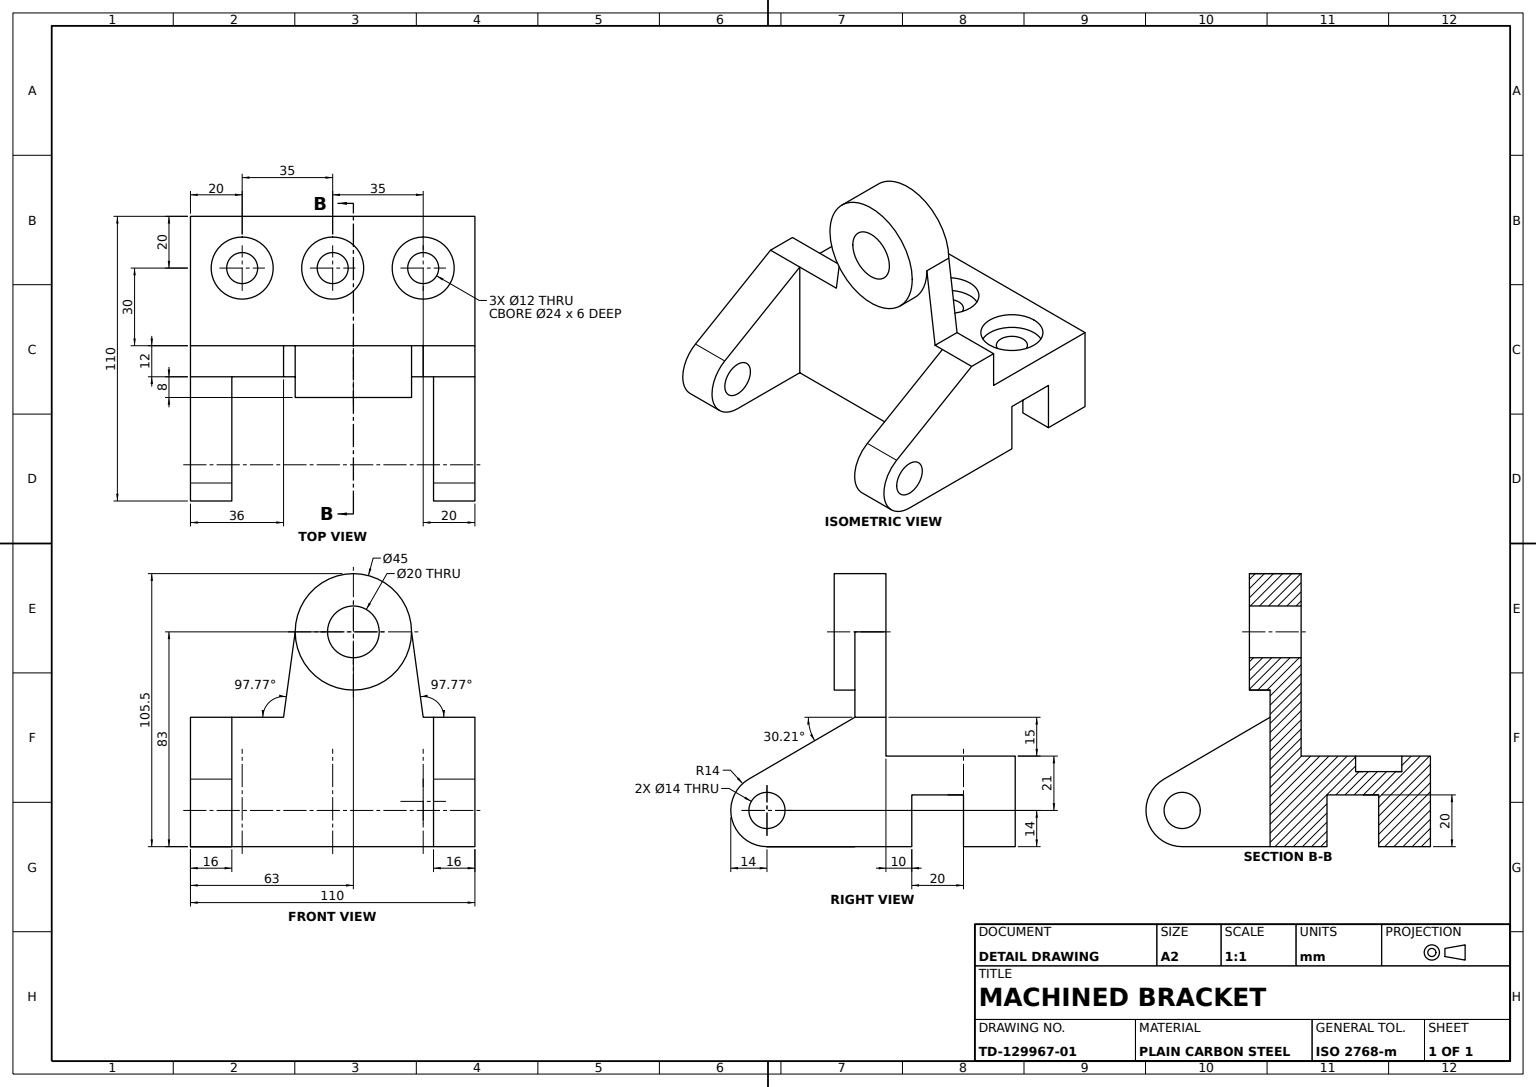
from build123d import *

# Parameters (mm, degrees)
SIDE_ARM_16MM_DEPTH          = 16
BRACKET_BODY_94MM_DEPTH      = 94
SECOND_START                 = -16
SECOND_ARM_16MM_DEPTH        = 16
PIVOT_HOLE_SKETCH_14_R       = 7
PIVOT_HOLES_14_THROUGH_DEPTH = 231
BEARING_BOSS_45_DEPTH        = 8
BEARING_BOSS_45_DEPTH_BACK   = 12
BEARING_BOSS_SKETCH_45_R     = 22.5
BOSS_SUPPORT_WEB_12MM_DEPTH  = 12
BEARING_BORE_SKETCH_20_R     = 10
BEARING_BORE_20_DEPTH        = 101
COUNTERBORE_SKETCH_24_R      = 12
COUNTERBORES_24X6_DEPTH      = 6
MOUNTING_HOLE_SKETCH_12_R    = 6
MOUNTING_HOLES_12_DEPTH      = 58


with BuildPart() as part:
    # Side Arm Profile → Side Arm 16mm (new body)
    with BuildSketch(Plane(origin=(0, 0, 0), x_dir=(0, 0, -1), z_dir=(1, 0, 0))):
        with BuildLine():
            Line((0, 0), (-20, 0))
            Line((-20, 0), (-20, 20))
            Line((-20, 20), (-40, 20))
            Line((-40, 20), (-40, 0))
            Line((-40, 0), (-96, 0))
            ThreePointArc((-96, 0), (-109.516186166, 10.351341133), (-103.045136072, 26.098184068))
            Line((-103.045136072, 26.098184068), (-62, 50))
            Line((-62, 50), (-50, 50))
            Line((-50, 50), (-50, 35))
            Line((-50, 35), (0, 35))
            Line((0, 35), (0, 0))
        make_face()
    extrude(amount=-SIDE_ARM_16MM_DEPTH)

    # Bracket Body Profile → Bracket Body 94mm (add)
    with BuildSketch(Plane.ZY.offset(16)):
        Polygon((0, 0), (0, 35), (50, 35), (50, 50), (62, 50), (62, 0), (40, 0), (40, 20), (20, 20), (20, 0), align=None)
    extrude(amount=BRACKET_BODY_94MM_DEPTH)

    # Second Arm Profile → Second Arm 16mm (add)
    with BuildSketch(Plane.ZY.offset(110).offset(SECOND_START)):
        with BuildLine():
            Line((62, 0), (62, 50))
            Line((62, 50), (103.045136072, 26.098184068))
            ThreePointArc((103.045136072, 26.098184068), (109.516186166, 10.351341133), (96, 0))
            Line((96, 0), (62, 0))
        make_face()
    extrude(amount=SECOND_ARM_16MM_DEPTH)

    # Pivot Hole Sketch Ø14 → Pivot Holes Ø14 Through (cut)
    with BuildSketch(Plane(origin=(0, 0, 0), x_dir=(0, 0, -1), z_dir=(1, 0, 0))):
        with Locations((-96, 14)):
            Circle(PIVOT_HOLE_SKETCH_14_R)
    extrude(amount=-PIVOT_HOLES_14_THROUGH_DEPTH, mode=Mode.SUBTRACT)



with BuildPart() as body_2:
    # Bearing Boss Sketch Ø45 → Bearing Boss Ø45 (new, two sides: drawn at the far end of the back side and taken through both)
    with BuildSketch(Plane.XY.offset(62).offset(-BEARING_BOSS_45_DEPTH_BACK)):
        with Locations((-47, 83)):
            Circle(BEARING_BOSS_SKETCH_45_R)
    extrude(amount=BEARING_BOSS_45_DEPTH + BEARING_BOSS_45_DEPTH_BACK)


with BuildPart() as part_1:
    add(part.part)

    add(body_2.part)  # Boss Support Web 12mm merges body 2
    # Boss Support Web Profile → Boss Support Web 12mm (add)
    with BuildSketch(Plane.XY.offset(62)):
        with BuildLine():
            Line((-20, 50), (-24.5, 83))
            ThreePointArc((-24.5, 83), (-47, 60.5), (-69.5, 83))
            Line((-69.5, 83), (-74, 50))
            Line((-74, 50), (-20, 50))
        make_face()
    extrude(amount=-BOSS_SUPPORT_WEB_12MM_DEPTH)

    # Bearing Bore Sketch Ø20 → Bearing Bore Ø20 (cut)
    with BuildSketch(Plane.XY.offset(70)):
        with Locations((-47, 83)):
            Circle(BEARING_BORE_SKETCH_20_R)
    extrude(amount=-BEARING_BORE_20_DEPTH, mode=Mode.SUBTRACT)

    # Counterbore Sketch Ø24 → Counterbores Ø24x6 (cut)
    with BuildSketch(Plane(origin=(0, 35, 0), x_dir=(1, 0, 0), z_dir=(0, 1, 0))):
        with Locations(Location((-20, -20, 0), (0, 0, 270))):
            Circle(COUNTERBORE_SKETCH_24_R)
        with Locations(Location((-55, -20, 0), (0, 0, 270))):
            Circle(COUNTERBORE_SKETCH_24_R)
        with Locations(Location((-90, -20, 0), (0, 0, 270))):
            Circle(COUNTERBORE_SKETCH_24_R)
    extrude(amount=-COUNTERBORES_24X6_DEPTH, mode=Mode.SUBTRACT)

    # Mounting Hole Sketch Ø12 → Mounting Holes Ø12 (cut)
    with BuildSketch(Plane(origin=(0, 29, 0), x_dir=(1, 0, 0), z_dir=(0, 1, 0))):
        with Locations(Location((-20, -20, 0), (0, 0, 270))):
            Circle(MOUNTING_HOLE_SKETCH_12_R)
        with Locations(Location((-55, -20, 0), (0, 0, 270))):
            Circle(MOUNTING_HOLE_SKETCH_12_R)
        with Locations(Location((-90, -20, 0), (0, 0, 270))):
            Circle(MOUNTING_HOLE_SKETCH_12_R)
    extrude(amount=-MOUNTING_HOLES_12_DEPTH, mode=Mode.SUBTRACT)


solid = part_1.part
